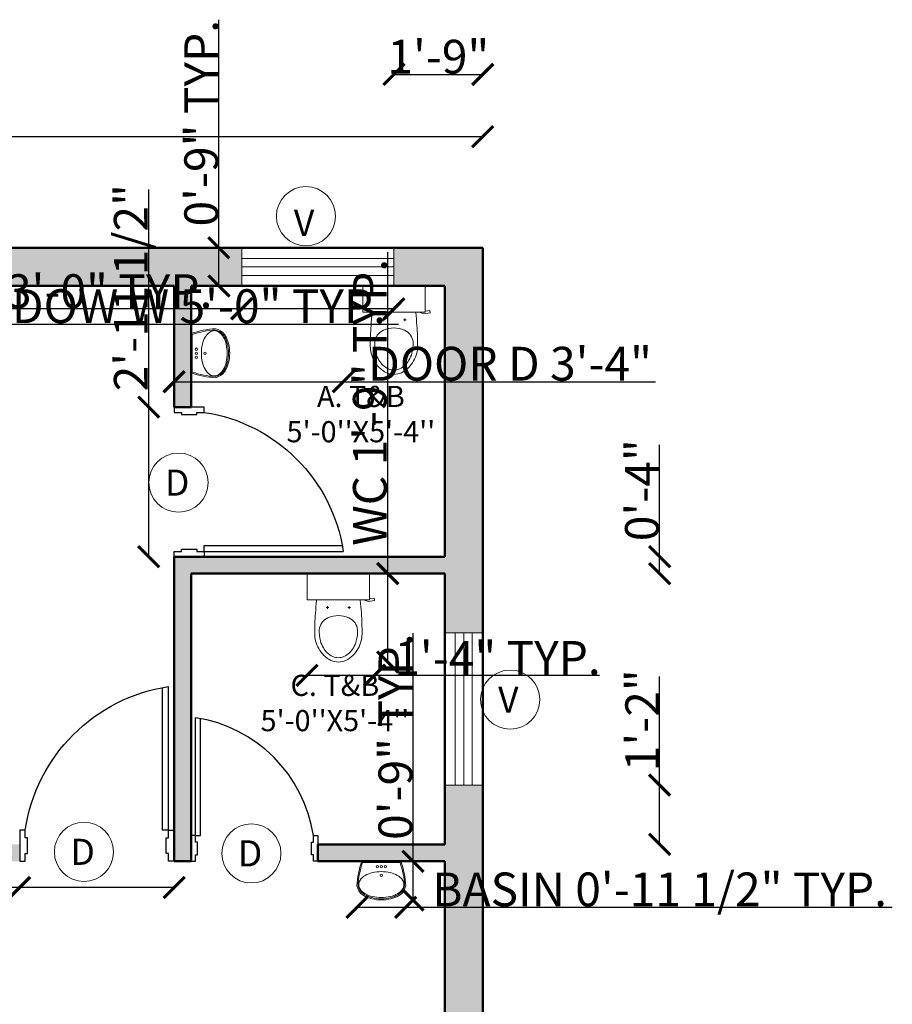
# Model space of a CAD drawing. Units: inches. Extents: x 1938 to 2373, y 1634 to 2225.
# Tile 5 of 5: x 2167 to 2373, y 1945 to 2178. Entities that reach past the tile are written whole.
import ezdxf

# ---------------------------------------------------------------- set-up
doc = ezdxf.new("R2010")
doc.units = ezdxf.units.IN
for name, color, linetype, lineweight in [('A-ANNO-DIMS', 2, 'Continuous', 18), ('A-ANNO-SYMB', 7, 'Continuous', 18), ('A-AREA-IDEN', 7, 'Continuous', 18), ('A-FLOR-FIXT', 9, 'Continuous', 18), ('A-WALL-PATT', 82, 'Continuous', 13), ('DOOR', 30, 'Continuous', 25), ('WALL', 7, 'Continuous', 50), ('WINDOW', 150, 'Continuous', 18)]:
    doc.layers.add(name, color=color, linetype=linetype, lineweight=lineweight)
doc.styles.get("Standard").update_dxf_attribs({"font": 'arial.ttf'})
doc.dimstyles.get("Standard").update_dxf_attribs({"dimtxt": 8, "dimasz": 5, "dimexe": 0.18, "dimexo": 0.0625, "dimgap": 0.09, "dimtad": 1, "dimdec": 1, "dimzin": 0, "dimdsep": 46, "dimlunit": 4, "dimtxsty": 'Standard', "dimblk": 'ARCHTICK', "dimcen": 0.09, "dimse1": 1, "dimse2": 1, "dimadec": 0, "dimazin": 0, "dimtfac": 1, "dimtdec": 1, "dimtofl": 0, "dimtmove": 0, "dimatfit": 3, "dimfxl": 1, "dimtolj": 1, "dimtzin": 0, "dimarcsym": 0})

# ---------------------------------------------------------------- blocks, each defined once
blk = doc.blocks.new('AP0B07')
for p, q in [((33.6, 96), (33.6, 978.8)), ((72, 96), (72, 972.3)), ((0, 96), (0, -96)), ((33.6, 96), (0, 96)), ((33.6, 48), (33.6, 96)), ((48, 48), (33.6, 48)), ((48, -48), (48, 48)), ((33.6, -96), (33.6, -48)), ((33.6, -48), (48, -48)), ((0, -96), (33.6, -96))]:
    blk.add_line(p, q)
blk.add_lwpolyline([(33.6, 96), (72, 96)])
blk.add_lwpolyline([(950, 96), (950, -96), (916.4, -96), (916.4, -48), (902, -48), (902, 48), (916.4, 48), (916.4, 96)], close=True)
blk.add_arc((-123.6, -61.2), 1051.8, 8.59637, 81.40363)
blk = doc.blocks.new('wash-3')
at = {"color": 0, "linetype": 'ByBlock'}
blk.add_line((0.23, -0.015), (-0.23, -0.015), dxfattribs=at)
for centre in [(-0.05, -0.066), (0, -0.066), (0.05, -0.066), (0, -0.172)]:
    blk.add_circle(centre, 0.0148, dxfattribs=at)
for centre, radius, start, end in [((0.69, -0.34), 0.991, 159.941, 177.839), ((0.69, -0.34), 0.976, 160.5399, 177.7326), ((-0.69, -0.34), 0.976, 2.2674, 19.4601), ((-0.69, -0.34), 0.991, 2.161, 20.059), ((-0.183, -0.286), 0.095, 144.1588, 180), ((-0.096, -0.349), 0.203, 119.8322, 144.1588), ((-0.038, -0.45), 0.319, 103.3619, 119.8322), ((0, -0.61), 0.483, 90, 103.3619), ((0, -0.61), 0.483, 76.6381, 90), ((0.038, -0.45), 0.319, 60.1678, 76.6381), ((0.096, -0.349), 0.203, 35.8412, 60.1678), ((0.183, -0.286), 0.095, 0, 35.8412), ((-0.12, -0.265), 0.184, 191.7424, 233.4191), ((-0.12, -0.265), 0.169, 192.3358, 233.361), ((-0.183, -0.286), 0.095, 180, 215.8412), ((-0.096, -0.223), 0.203, 215.8412, 240.1678), ((0.096, -0.223), 0.203, 299.8322, 324.1588), ((0.12, -0.265), 0.169, 306.639, 347.6642), ((0.12, -0.265), 0.184, 306.5809, 348.2576), ((0.183, -0.286), 0.095, 324.1588, 0), ((-0.096, -0.223), 0.232, 234.7719, 240.1678), ((-0.096, -0.223), 0.217, 234.8176, 240.1678), ((-0.038, -0.122), 0.348, 240.1678, 256.6381), ((-0.038, -0.122), 0.333, 240.1678, 256.6381), ((-0.038, -0.122), 0.319, 240.1678, 256.6381), ((0, 0.038), 0.513, 256.6381, 270), ((0, 0.038), 0.498, 256.6381, 270), ((0, 0.038), 0.483, 256.6381, 270), ((0, 0.038), 0.483, 270, 283.3619), ((0, 0.038), 0.498, 270, 283.3619), ((0, 0.038), 0.513, 270, 283.3619), ((0.038, -0.122), 0.319, 283.3619, 299.8322), ((0.038, -0.122), 0.333, 283.3619, 299.8322), ((0.038, -0.122), 0.348, 283.3619, 299.8322), ((0.096, -0.223), 0.217, 299.8322, 305.1824), ((0.096, -0.223), 0.232, 299.8322, 305.2281)]:
    blk.add_arc(centre, radius, start, end, dxfattribs=at)
blk = doc.blocks.new('toilet-1')
at = {"color": 0, "linetype": 'ByBlock'}
for p, q in [((-0.23, -0.02), (-0.23, -0.2116)), ((0.23, -0.02), (-0.23, -0.02)), ((0.23, -0.02), (0.23, -0.2116)), ((-0.23, -0.2116), (0.23, -0.2116)), ((0.1917, -0.2144), (0.2206, -0.225)), ((0.2633, -0.1997), (0.23, -0.2044)), ((0.266, -0.2187), (0.2633, -0.1997)), ((-0.0889, -0.2683), (-0.0697, -0.2683)), ((-0.0793, -0.2587), (-0.0793, -0.2778)), ((0.0889, -0.2683), (0.0698, -0.2683)), ((0.0794, -0.2587), (0.0794, -0.2778)), ((0.2206, -0.225), (0.266, -0.2187)), ((0, -0.6382), (0, -0.6382))]:
    blk.add_line(p, q, dxfattribs=at)
for centre, radius, start, end in [((3.5272, -0.6239), 3.7093, 173.69251, 175.15926), ((-3.527, -0.624), 3.7093, 4.84131, 6.31706), ((1.7368, -0.4519), 1.9109, 175.76982, 180.37578), ((-0.0312, -0.4465), 0.1114, 113.89968, 145.1485), ((0, -0.5169), 0.1884, 66.09393, 113.90607), ((0.0312, -0.4465), 0.1114, 34.8515, 66.10032), ((-1.7366, -0.4519), 1.9109, 359.62422, 4.23018), ((0.0981, -0.4497), 0.2389, 175.88621, 195.59308), ((-0.0408, -0.4398), 0.0996, 145.14967, 175.88096), ((0.0409, -0.4398), 0.0996, 4.11904, 34.85033), ((-0.098, -0.4497), 0.2389, 344.40692, 4.11379), ((0.0353, -0.463), 0.2093, 180.37466, 194.33753), ((-0.0351, -0.463), 0.2093, 345.6614, 359.62427), ((0.055, -0.458), 0.2297, 194.33532, 209.62204), ((0.0647, -0.4524), 0.2409, 209.62726, 224.54888), ((0.0961, -0.4503), 0.2369, 195.59686, 209.37705), ((0.0232, -0.4913), 0.1532, 209.38715, 226.54376), ((-0.0231, -0.4913), 0.1532, 313.45624, 330.61285), ((-0.0645, -0.4524), 0.2409, 315.45042, 330.37204), ((-0.096, -0.4503), 0.2369, 330.62295, 344.40314), ((-0.0548, -0.458), 0.2297, 330.37879, 345.66551), ((0.0178, -0.4986), 0.1751, 224.55199, 245.714), ((0.0152, -0.4997), 0.1416, 226.55015, 246.55272), ((0, -0.5347), 0.1034, 246.54933, 270.0042), ((0, -0.5347), 0.1034, 269.9958, 293.45067), ((-0.0151, -0.4997), 0.1416, 293.44728, 313.44985), ((-0.0176, -0.4986), 0.1751, 294.28649, 315.4485), ((0.0004, -0.538), 0.132, 245.58449, 269.87817), ((-0.0002, -0.538), 0.132, 270.12162, 294.4153)]:
    blk.add_arc(centre, radius, start, end, dxfattribs=at)
blk = doc.blocks.new('_ArchTick')
at = {"color": 0, "linetype": 'ByBlock', "const_width": 0.15}
blk.add_lwpolyline([(-0.5, -0.5), (0.5, 0.5)], dxfattribs=at)
blk = doc.blocks.new('*D12')
at = {"layer": 'A-ANNO-DIMS', "color": 0, "lineweight": -2, "transparency": 16777216}
blk.add_line((2000.23, 2149.88), (2276.23, 2149.88), dxfattribs=at)
at = {"layer": 'Defpoints', "color": 0, "transparency": 16777216}
for p in [(2276.23, 2149.88), (2000.23, 2123.59), (2276.23, 2123.59)]:
    blk.add_point(p, dxfattribs=at)
at = {"layer": 'A-ANNO-DIMS', "color": 0, "lineweight": -2, "transparency": 16777216, "xscale": 5, "yscale": 5, "zscale": 5, "rotation": 180}
blk.add_blockref('_ArchTick', (2000.23, 2149.88), dxfattribs=at)
at = {"layer": 'A-ANNO-DIMS', "color": 0, "lineweight": -2, "transparency": 16777216, "xscale": 5, "yscale": 5, "zscale": 5}
blk.add_blockref('_ArchTick', (2276.23, 2149.88), dxfattribs=at)
at = {"layer": 'A-ANNO-DIMS', "color": 0, "transparency": 16777216, "insert": (2138.23, 2154.06), "char_height": 8, "attachment_point": 5}
blk.add_mtext("\\A1;23'", dxfattribs=at)
blk = doc.blocks.new('VENT-36IN')
for p, q in [((2.5, 36), (2.5, 0)), ((4.5, 36), (4.5, 0)), ((6.5, 36), (6.5, 0))]:
    blk.add_line(p, q)
blk.add_lwpolyline([(9, 36), (0, 36), (0, 0), (9, 0)], close=True)
blk = doc.blocks.new('TAG-DOOR-D')
blk.add_circle((7, 7), 7)
blk.add_text('D', height=6.17).set_placement((3.79, 3.92))
blk = doc.blocks.new('*D21')
at = {"layer": 'A-ANNO-DIMS', "color": 0, "lineweight": -2, "transparency": 16777216}
for p, q in [((2160.51, 2019.91), (2160.51, 2112.41)), ((2160.51, 1978.59), (2160.51, 2019.91))]:
    blk.add_line(p, q, dxfattribs=at)
at = {"layer": 'Defpoints', "color": 0, "transparency": 16777216}
for p in [(2160.51, 2019.91), (2166.7, 2019.91), (2166.7, 1978.59)]:
    blk.add_point(p, dxfattribs=at)
at = {"layer": 'A-ANNO-DIMS', "color": 0, "lineweight": -2, "transparency": 16777216, "xscale": 5, "yscale": 5, "zscale": 5}
for p, rotation in [((2160.51, 2019.91), 90), ((2160.51, 1978.59), 270)]:
    blk.add_blockref('_ArchTick', p, dxfattribs=dict(at, rotation=rotation))
at = {"layer": 'A-ANNO-DIMS', "color": 0, "transparency": 16777216, "insert": (2156.27, 2068.66), "char_height": 8, "attachment_point": 5, "rotation": 90}
blk.add_mtext('\\A1;DOOR D 3\'-5 1/2"', dxfattribs=at)
blk = doc.blocks.new('*D22')
at = {"layer": 'A-ANNO-DIMS', "color": 0, "lineweight": -2, "transparency": 16777216}
for p, q in [((2166.7, 1972.39), (2121.62, 1972.39)), ((2203.23, 1972.39), (2166.7, 1972.39))]:
    blk.add_line(p, q, dxfattribs=at)
at = {"layer": 'Defpoints', "color": 0, "transparency": 16777216}
for p in [(2166.7, 1978.59), (2203.23, 1978.59), (2166.7, 1972.39)]:
    blk.add_point(p, dxfattribs=at)
at = {"layer": 'A-ANNO-DIMS', "color": 0, "lineweight": -2, "transparency": 16777216, "xscale": 5, "yscale": 5, "zscale": 5, "rotation": 180}
blk.add_blockref('_ArchTick', (2166.7, 1972.39), dxfattribs=at)
at = {"layer": 'A-ANNO-DIMS', "color": 0, "lineweight": -2, "transparency": 16777216, "xscale": 5, "yscale": 5, "zscale": 5}
blk.add_blockref('_ArchTick', (2203.23, 1972.39), dxfattribs=at)
at = {"layer": 'A-ANNO-DIMS', "color": 0, "transparency": 16777216, "insert": (2141.66, 1976.62), "char_height": 8, "attachment_point": 5}
blk.add_mtext('\\A1;3\'-0 1/2"', dxfattribs=at)
blk = doc.blocks.new('*D23')
at = {"layer": 'A-ANNO-DIMS', "color": 0, "lineweight": -2, "transparency": 16777216}
for p, q in [((2203.23, 2091.96), (2243.25, 2091.96)), ((2243.25, 2091.96), (2317.11, 2091.96))]:
    blk.add_line(p, q, dxfattribs=at)
at = {"layer": 'Defpoints', "color": 0, "transparency": 16777216}
for p in [(2243.25, 2091.96), (2203.23, 2085.96), (2243.25, 2085.96)]:
    blk.add_point(p, dxfattribs=at)
at = {"layer": 'A-ANNO-DIMS', "color": 0, "lineweight": -2, "transparency": 16777216, "xscale": 5, "yscale": 5, "zscale": 5, "rotation": 180}
blk.add_blockref('_ArchTick', (2203.23, 2091.96), dxfattribs=at)
at = {"layer": 'A-ANNO-DIMS', "color": 0, "lineweight": -2, "transparency": 16777216, "xscale": 5, "yscale": 5, "zscale": 5}
blk.add_blockref('_ArchTick', (2243.25, 2091.96), dxfattribs=at)
at = {"layer": 'A-ANNO-DIMS', "color": 0, "transparency": 16777216, "insert": (2282.68, 2096.2), "char_height": 8, "attachment_point": 5}
blk.add_mtext('\\A1;DOOR D 3\'-4"', dxfattribs=at)
blk = doc.blocks.new('*D24')
at = {"layer": 'A-ANNO-DIMS', "color": 0, "lineweight": -2, "transparency": 16777216}
for p, q in [((2197.23, 2085.96), (2197.23, 2137.4)), ((2197.23, 2050.59), (2197.23, 2085.96))]:
    blk.add_line(p, q, dxfattribs=at)
at = {"layer": 'Defpoints', "color": 0, "transparency": 16777216}
for p in [(2197.23, 2085.96), (2203.23, 2085.96), (2203.23, 2050.59)]:
    blk.add_point(p, dxfattribs=at)
at = {"layer": 'A-ANNO-DIMS', "color": 0, "lineweight": -2, "transparency": 16777216, "xscale": 5, "yscale": 5, "zscale": 5}
for p, rotation in [((2197.23, 2085.96), 90), ((2197.23, 2050.59), 270)]:
    blk.add_blockref('_ArchTick', p, dxfattribs=dict(at, rotation=rotation))
at = {"layer": 'A-ANNO-DIMS', "color": 0, "transparency": 16777216, "insert": (2193, 2114.18), "char_height": 8, "attachment_point": 5, "rotation": 90}
blk.add_mtext('\\A1;2\'-11 1/2"', dxfattribs=at)
blk = doc.blocks.new('*D29')
at = {"layer": 'A-ANNO-DIMS', "color": 0, "lineweight": -2, "transparency": 16777216}
for p, q in [((2076.23, 2105.59), (2136.23, 2105.59)), ((2136.23, 2105.59), (2256.3, 2105.59))]:
    blk.add_line(p, q, dxfattribs=at)
at = {"layer": 'Defpoints', "color": 0, "transparency": 16777216}
for p in [(2076.23, 2114.59), (2136.23, 2114.59), (2136.23, 2105.59)]:
    blk.add_point(p, dxfattribs=at)
at = {"layer": 'A-ANNO-DIMS', "color": 0, "lineweight": -2, "transparency": 16777216, "xscale": 5, "yscale": 5, "zscale": 5, "rotation": 180}
blk.add_blockref('_ArchTick', (2076.23, 2105.59), dxfattribs=at)
at = {"layer": 'A-ANNO-DIMS', "color": 0, "lineweight": -2, "transparency": 16777216, "xscale": 5, "yscale": 5, "zscale": 5}
blk.add_blockref('_ArchTick', (2136.23, 2105.59), dxfattribs=at)
at = {"layer": 'A-ANNO-DIMS', "color": 0, "transparency": 16777216, "insert": (2198.76, 2109.81), "char_height": 8, "attachment_point": 5}
blk.add_mtext('\\A1;WINDOW W 5\'-0" TYP.', dxfattribs=at)
blk = doc.blocks.new('*D33')
at = {"layer": 'A-ANNO-DIMS', "color": 0, "lineweight": -2, "transparency": 16777216}
for p, q in [((2246.47, 1967.71), (2258.01, 1967.71)), ((2258.01, 1967.71), (2373.1, 1967.71))]:
    blk.add_line(p, q, dxfattribs=at)
at = {"layer": 'Defpoints', "color": 0, "transparency": 16777216}
for p in [(2246.47, 1969.44), (2258.01, 1969.44), (2258.01, 1967.71)]:
    blk.add_point(p, dxfattribs=at)
at = {"layer": 'A-ANNO-DIMS', "color": 0, "lineweight": -2, "transparency": 16777216, "xscale": 5, "yscale": 5, "zscale": 5, "rotation": 180}
blk.add_blockref('_ArchTick', (2246.47, 1967.71), dxfattribs=at)
at = {"layer": 'A-ANNO-DIMS', "color": 0, "lineweight": -2, "transparency": 16777216, "xscale": 5, "yscale": 5, "zscale": 5}
blk.add_blockref('_ArchTick', (2258.01, 1967.71), dxfattribs=at)
at = {"layer": 'A-ANNO-DIMS', "color": 0, "transparency": 16777216, "insert": (2318.06, 1971.94), "char_height": 8, "attachment_point": 5}
blk.add_mtext('\\A1;BASIN 0\'-11 1/2" TYP.', dxfattribs=at)
blk = doc.blocks.new('*D34')
at = {"layer": 'A-ANNO-DIMS', "color": 0, "lineweight": -2, "transparency": 16777216}
for p, q in [((2259.74, 1978.59), (2259.74, 2032.53)), ((2259.74, 1969.44), (2259.74, 1978.59))]:
    blk.add_line(p, q, dxfattribs=at)
at = {"layer": 'Defpoints', "color": 0, "transparency": 16777216}
for p in [(2258.01, 1978.59), (2259.74, 1978.59), (2258.01, 1969.44)]:
    blk.add_point(p, dxfattribs=at)
at = {"layer": 'A-ANNO-DIMS', "color": 0, "lineweight": -2, "transparency": 16777216, "xscale": 5, "yscale": 5, "zscale": 5}
for p, rotation in [((2259.74, 1978.59), 90), ((2259.74, 1969.44), 270)]:
    blk.add_blockref('_ArchTick', p, dxfattribs=dict(at, rotation=rotation))
at = {"layer": 'A-ANNO-DIMS', "color": 0, "transparency": 16777216, "insert": (2255.57, 2008.06), "char_height": 8, "attachment_point": 5, "rotation": 90}
blk.add_mtext('\\A1;0\'-9" TYP.', dxfattribs=at)
blk = doc.blocks.new('*D37')
at = {"layer": 'A-ANNO-DIMS', "color": 0, "lineweight": -2, "transparency": 16777216}
for p, q in [((2253.76, 2046.59), (2253.76, 2122.58)), ((2253.76, 2025.69), (2253.76, 2046.59))]:
    blk.add_line(p, q, dxfattribs=at)
at = {"layer": 'Defpoints', "color": 0, "transparency": 16777216}
for p in [(2250.63, 2046.59), (2253.76, 2046.59), (2250.63, 2025.69)]:
    blk.add_point(p, dxfattribs=at)
at = {"layer": 'A-ANNO-DIMS', "color": 0, "lineweight": -2, "transparency": 16777216, "xscale": 5, "yscale": 5, "zscale": 5}
for p, rotation in [((2253.76, 2046.59), 90), ((2253.76, 2025.69), 270)]:
    blk.add_blockref('_ArchTick', p, dxfattribs=dict(at, rotation=rotation))
at = {"layer": 'A-ANNO-DIMS', "color": 0, "transparency": 16777216, "insert": (2249.54, 2087.08), "char_height": 8, "attachment_point": 5, "rotation": 90}
blk.add_mtext('\\A1;WC 1\'-9" TYP.', dxfattribs=at)
blk = doc.blocks.new('*D38')
at = {"layer": 'A-ANNO-DIMS', "color": 0, "lineweight": -2, "transparency": 16777216}
for p, q in [((2234.68, 2022.55), (2250.63, 2022.55)), ((2250.63, 2022.55), (2303.82, 2022.55))]:
    blk.add_line(p, q, dxfattribs=at)
at = {"layer": 'Defpoints', "color": 0, "transparency": 16777216}
for p in [(2234.68, 2025.69), (2250.63, 2025.69), (2250.63, 2022.55)]:
    blk.add_point(p, dxfattribs=at)
at = {"layer": 'A-ANNO-DIMS', "color": 0, "lineweight": -2, "transparency": 16777216, "xscale": 5, "yscale": 5, "zscale": 5, "rotation": 180}
blk.add_blockref('_ArchTick', (2234.68, 2022.55), dxfattribs=at)
at = {"layer": 'A-ANNO-DIMS', "color": 0, "lineweight": -2, "transparency": 16777216, "xscale": 5, "yscale": 5, "zscale": 5}
blk.add_blockref('_ArchTick', (2250.63, 2022.55), dxfattribs=at)
at = {"layer": 'A-ANNO-DIMS', "color": 0, "transparency": 16777216, "insert": (2279.72, 2026.66), "char_height": 8, "attachment_point": 5}
blk.add_mtext('\\A1;1\'-4" TYP.', dxfattribs=at)
blk = doc.blocks.new('*D41')
at = {"layer": 'A-ANNO-DIMS', "color": 0, "lineweight": -2, "transparency": 16777216}
for p, q in [((2219.23, 2109.19), (2131.96, 2109.19)), ((2255.23, 2109.19), (2219.23, 2109.19))]:
    blk.add_line(p, q, dxfattribs=at)
at = {"layer": 'Defpoints', "color": 0, "transparency": 16777216}
for p in [(2219.23, 2114.59), (2255.23, 2114.59), (2219.23, 2109.19)]:
    blk.add_point(p, dxfattribs=at)
at = {"layer": 'A-ANNO-DIMS', "color": 0, "lineweight": -2, "transparency": 16777216, "xscale": 5, "yscale": 5, "zscale": 5}
for p, rotation in [((2219.23, 2109.19), 179.9999999999986), ((2255.23, 2109.19), 359.9999999999986)]:
    blk.add_blockref('_ArchTick', p, dxfattribs=dict(at, rotation=rotation))
at = {"layer": 'A-ANNO-DIMS', "color": 0, "transparency": 16777216, "insert": (2173.09, 2113.36), "char_height": 8, "attachment_point": 5}
blk.add_mtext('\\A1;VENT 3\'-0" TYP.', dxfattribs=at)
blk = doc.blocks.new('*D42')
at = {"layer": 'A-ANNO-DIMS', "color": 0, "lineweight": -2, "transparency": 16777216}
for p, q in [((2213.83, 2123.59), (2213.83, 2177.53)), ((2213.83, 2114.59), (2213.83, 2123.59))]:
    blk.add_line(p, q, dxfattribs=at)
at = {"layer": 'Defpoints', "color": 0, "transparency": 16777216}
for p in [(2213.83, 2123.59), (2219.23, 2123.59), (2219.23, 2114.59)]:
    blk.add_point(p, dxfattribs=at)
at = {"layer": 'A-ANNO-DIMS', "color": 0, "lineweight": -2, "transparency": 16777216, "xscale": 5, "yscale": 5, "zscale": 5}
for p, rotation in [((2213.83, 2123.59), 90), ((2213.83, 2114.59), 270)]:
    blk.add_blockref('_ArchTick', p, dxfattribs=dict(at, rotation=rotation))
at = {"layer": 'A-ANNO-DIMS', "color": 0, "transparency": 16777216, "insert": (2209.65, 2153.06), "char_height": 8, "attachment_point": 5, "rotation": 90}
blk.add_mtext('\\A1;0\'-9" TYP.', dxfattribs=at)
blk = doc.blocks.new('*D59')
at = {"layer": 'A-ANNO-DIMS', "color": 0, "lineweight": -2, "transparency": 16777216}
blk.add_line((2255.23, 2164.6), (2276.23, 2164.6), dxfattribs=at)
at = {"layer": 'Defpoints', "color": 0, "transparency": 16777216}
for p in [(2276.23, 2164.6), (2255.23, 2123.59), (2276.23, 2123.59)]:
    blk.add_point(p, dxfattribs=at)
at = {"layer": 'A-ANNO-DIMS', "color": 0, "lineweight": -2, "transparency": 16777216, "xscale": 5, "yscale": 5, "zscale": 5, "rotation": 180}
blk.add_blockref('_ArchTick', (2255.23, 2164.6), dxfattribs=at)
at = {"layer": 'A-ANNO-DIMS', "color": 0, "lineweight": -2, "transparency": 16777216, "xscale": 5, "yscale": 5, "zscale": 5}
blk.add_blockref('_ArchTick', (2276.23, 2164.6), dxfattribs=at)
at = {"layer": 'A-ANNO-DIMS', "color": 0, "transparency": 16777216, "insert": (2265.73, 2168.77), "char_height": 8, "attachment_point": 5}
blk.add_mtext('\\A1;1\'-9"', dxfattribs=at)
blk = doc.blocks.new('*D64')
at = {"layer": 'A-ANNO-DIMS', "color": 0, "lineweight": -2, "transparency": 16777216}
for p, q in [((2318.07, 1996.59), (2318.07, 2022.28)), ((2318.07, 1982.59), (2318.07, 1996.59))]:
    blk.add_line(p, q, dxfattribs=at)
at = {"layer": 'Defpoints', "color": 0, "transparency": 16777216}
for p in [(2267.23, 1996.59), (2318.07, 1996.59), (2267.23, 1982.59)]:
    blk.add_point(p, dxfattribs=at)
at = {"layer": 'A-ANNO-DIMS', "color": 0, "lineweight": -2, "transparency": 16777216, "xscale": 5, "yscale": 5, "zscale": 5}
for p, rotation in [((2318.07, 1996.59), 90), ((2318.07, 1982.59), 270)]:
    blk.add_blockref('_ArchTick', p, dxfattribs=dict(at, rotation=rotation))
at = {"layer": 'A-ANNO-DIMS', "color": 0, "transparency": 16777216, "insert": (2313.96, 2011.93), "char_height": 8, "attachment_point": 5, "rotation": 90}
blk.add_mtext('\\A1;1\'-2"', dxfattribs=at)
blk = doc.blocks.new('*D66')
at = {"layer": 'A-ANNO-DIMS', "color": 0, "lineweight": -2, "transparency": 16777216}
for p, q in [((2318.07, 2050.59), (2318.07, 2077.03)), ((2318.07, 2046.59), (2318.07, 2050.59))]:
    blk.add_line(p, q, dxfattribs=at)
at = {"layer": 'Defpoints', "color": 0, "transparency": 16777216}
for p in [(2267.23, 2050.59), (2318.07, 2050.59), (2267.23, 2046.59)]:
    blk.add_point(p, dxfattribs=at)
at = {"layer": 'A-ANNO-DIMS', "color": 0, "lineweight": -2, "transparency": 16777216, "xscale": 5, "yscale": 5, "zscale": 5}
for p, rotation in [((2318.07, 2050.59), 90), ((2318.07, 2046.59), 270)]:
    blk.add_blockref('_ArchTick', p, dxfattribs=dict(at, rotation=rotation))
at = {"layer": 'A-ANNO-DIMS', "color": 0, "transparency": 16777216, "insert": (2313.89, 2066.31), "char_height": 8, "attachment_point": 5, "rotation": 90}
blk.add_mtext('\\A1;0\'-4"', dxfattribs=at)

msp = doc.modelspace()

# ---------------------------------------------------------------- hatches: boundary and pattern name
at = {"layer": 'A-WALL-PATT', "transparency": 33554585}
h = msp.add_hatch(color=256, dxfattribs=at)
h.dxf.hatch_style = 1
h.paths.add_polyline_path([(2076.23, 2123.59), (2000.23, 2123.59), (2000.23, 2078.59), (2009.23, 2078.59), (2009.23, 2078.85), (2009.23, 2114.59), (2076.23, 2114.59)])
h.paths.add_polyline_path([(2219.23, 2123.59), (2136.23, 2123.59), (2136.23, 2114.59), (2203.23, 2114.59), (2203.23, 2085.96), (2207.23, 2085.96), (2207.23, 2114.59), (2219.23, 2114.59)])
h.paths.add_polyline_path([(2276.23, 2123.59), (2255.23, 2123.59), (2255.23, 2114.59), (2262.62, 2114.59), (2267.23, 2114.59), (2267.23, 2050.59), (2203.23, 2050.59), (2203.23, 1978.59), (2207.23, 1978.59), (2207.23, 1984.65), (2207.23, 2046.59), (2267.23, 2046.59), (2267.23, 2032.59), (2276.23, 2032.59)])
h.paths.add_polyline_path([(2009.23, 2018.59), (2000.23, 2018.59), (2000.23, 1948.59), (2009.23, 1948.59), (2009.23, 1948.85), (2009.23, 1978.59), (2126.4, 1978.59), (2126.4, 1978.59), (2133.23, 1978.59), (2166.7, 1978.59), (2166.7, 1982.59), (2009.23, 1982.59)])
h.paths.add_polyline_path([(2276.23, 1996.59), (2267.23, 1996.59), (2267.23, 1982.59), (2237.23, 1982.59), (2237.23, 1978.59), (2267.23, 1978.59), (2267.23, 1901.32), (2276.23, 1901.32)])
h.paths.add_polyline_path([(2133.23, 1944.79), (2129.23, 1944.79), (2129.23, 1858.59), (2009.23, 1858.59), (2009.23, 1888.59), (2000.23, 1888.59), (2000.23, 1839.09), (2009.23, 1839.09), (2009.23, 1854.59), (2091.31, 1854.59), (2091.31, 1854.61), (2097.36, 1854.59), (2133.23, 1854.59)])
h.paths.add_polyline_path([(2121.02, 1763.59), (2097.23, 1763.59), (2097.23, 1824.61), (2093.23, 1824.61), (2093.23, 1763.59), (2009.23, 1763.59), (2009.23, 1779.09), (2000.23, 1779.09), (2000.23, 1739.59), (2009.23, 1739.59), (2009.23, 1754.59), (2121.02, 1754.59)])
h.paths.add_polyline_path([(2108.23, 1676.59), (2009.23, 1676.59), (2009.23, 1691.59), (2000.23, 1691.59), (2000.23, 1667.59), (2108.23, 1667.59)])
h.paths.add_polyline_path([(2276.23, 1841.32), (2267.23, 1841.32), (2267.23, 1763.59), (2246.64, 1763.59), (2246.64, 1754.59), (2276.23, 1754.59)])

# ---------------------------------------------------------------- linework, layer by layer
at = {"layer": 'A-ANNO-SYMB'}
for centre in [(2234.41, 2131.07), (2282.72, 2016.8)]:
    msp.add_circle(centre, 7, dxfattribs=at)
at = {"layer": 'WALL'}
for p, q in [((2000.23, 2123.59), (2276.23, 2123.59)), ((2276.23, 2123.59), (2276.23, 1667.59)), ((2009.23, 2114.59), (2203.23, 2114.59)), ((2203.23, 2114.59), (2203.23, 2085.96)), ((2207.23, 2114.59), (2207.23, 2085.96)), ((2207.23, 2114.59), (2267.23, 2114.59)), ((2267.23, 2114.59), (2267.23, 2050.59)), ((2203.23, 2085.96), (2207.23, 2085.96)), ((2203.23, 2050.59), (2267.23, 2050.59)), ((2203.23, 2050.59), (2203.23, 1978.59)), ((2207.23, 2046.59), (2267.23, 2046.59)), ((2207.23, 2046.59), (2207.23, 1978.59)), ((2267.23, 2046.59), (2267.23, 1982.59)), ((2237.23, 1982.59), (2267.23, 1982.59)), ((2237.23, 1982.59), (2237.23, 1978.59)), ((2203.23, 1978.59), (2207.23, 1978.59)), ((2237.23, 1978.59), (2267.23, 1978.59)), ((2267.23, 1763.59), (2267.23, 1978.59))]:
    msp.add_line(p, q, dxfattribs=at)

# ---------------------------------------------------------------- block references
at = {"layer": 'A-ANNO-SYMB'}
for p in [(2197.27, 2061.1), (2174.91, 1973.82), (2214.5, 1973.46)]:
    msp.add_blockref('TAG-DOOR-D', p, dxfattribs=at)
at = {"layer": 'A-FLOR-FIXT'}
for name, p, xscale, yscale, zscale in [('toilet-1', (2255.23, 2115.23), 32.14984283332795, 32.14984283332795, 32.14984283332795), ('toilet-1', (2242.08, 2047.23), 32.14984283332795, 32.14984283332795, 32.14984283332795), ('wash-3', (2252.24, 1978.59), 19.24466160509284, 19.24466160509284, 19.24466160509284)]:
    msp.add_blockref(name, p, dxfattribs=dict(at, xscale=xscale, yscale=yscale, zscale=zscale))
at = {"layer": 'A-FLOR-FIXT', "xscale": 19.24466160509284, "yscale": 19.24466160509284, "zscale": 19.24466160509284, "rotation": 90}
msp.add_blockref('wash-3', (2207.23, 2098.68), dxfattribs=at)
at = {"layer": 'DOOR', "xscale": -0.0372377324197297, "yscale": 0.0372377324197297, "zscale": 0.0372377324197297, "rotation": 270}
msp.add_blockref('AP0B07', (2206.8, 2050.59), dxfattribs=at)
at = {"layer": 'DOOR'}
for p, xscale, yscale, zscale in [((2203.23, 1982.28), -0.0384472811899697, 0.0384472811899697, 0.0384472811899697), ((2207.23, 1981.62), 0.031578947368421, 0.031578947368421, 0.031578947368421)]:
    msp.add_blockref('AP0B07', p, dxfattribs=dict(at, xscale=xscale, yscale=yscale, zscale=zscale))
at = {"layer": 'WINDOW', "rotation": 89.99999999999844}
msp.add_blockref('VENT-36IN', (2255.23, 2114.59), dxfattribs=at)
at = {"layer": 'WINDOW'}
msp.add_blockref('VENT-36IN', (2267.23, 1996.59), dxfattribs=at)

# ---------------------------------------------------------------- texts
at = {"layer": 'A-ANNO-SYMB'}
for p in [(2231.55, 2126.42), (2279.86, 2013.72)]:
    msp.add_text('V', height=6.17, dxfattribs=at).set_placement(p)
at = {"layer": 'A-AREA-IDEN', "char_height": 5, "attachment_point": 1}
for s, insert in [("\\pxi-3,l4,qc,t4;A. T&B\\P5'-0''X5'-4''", (2213.15, 2090.97)), ("\\pxqc;C. T&B\\P5'-0''X5'-4''", (2209.5, 2022.68))]:
    msp.add_mtext_dynamic_manual_height_columns(s, width=63.5129, gutter_width=30.83, heights=[0], dxfattribs=dict(at, insert=insert))

# ---------------------------------------------------------------- dimensions: what is measured, and where the dimension line sits
at = {"layer": 'A-ANNO-DIMS'}
for base, p1, p2, angle, text, picture, middle in [((2213.83, 2123.59), (2219.23, 2114.59), (2219.23, 2123.59), 90, '<> TYP.', '*D42', (2209.65, 2153.06)), ((2136.23, 2105.59), (2076.23, 2114.59), (2136.23, 2114.59), 0, 'WINDOW W <> TYP.', '*D29', (2198.76, 2109.81)), ((2219.23, 2109.19), (2255.23, 2114.59), (2219.23, 2114.59), 180, 'VENT <> TYP.', '*D41', (2173.09, 2113.36)), ((2253.76, 2046.59), (2250.63, 2025.69), (2250.63, 2046.59), 90, 'WC <> TYP.', '*D37', (2249.54, 2087.08)), ((2160.51, 2019.91), (2166.7, 1978.59), (2166.7, 2019.91), 90, 'DOOR D <>', '*D21', (2156.27, 2068.66)), ((2259.7448, 1978.5853), (2258.0127, 1969.444), (2258.0127, 1978.5853), 90, '<> TYP.', '*D34', (2255.5702, 2008.0573))]:
    dim = msp.add_linear_dim(base=base, p1=p1, p2=p2, angle=angle, text=text, dimstyle='Standard', override={"dimdec": 1, "dimlfac": 1, "dimrnd": 0, "dimzin": 1, "dimdsep": 46, "dimlunit": 4, "dimfrac": 2}, dxfattribs=at)
    dim.commit()
    dim.dimension.update_dxf_attribs({"geometry": picture, "text_midpoint": middle})
for base, p1, override, picture, middle in [((2276.23, 2164.6), (2255.23, 2123.59), {"dimdec": 1, "dimlfac": 1, "dimrnd": 0, "dimzin": 1, "dimdsep": 46, "dimlunit": 4, "dimfrac": 2}, '*D59', (2265.73, 2168.77)), ((2276.23, 2149.88), (2000.23, 2123.59), {"dimclrd": 0, "dimclre": 0, "dimclrt": 0}, '*D12', (2138.23, 2154.06))]:
    dim = msp.add_linear_dim(base=base, p1=p1, p2=(2276.23, 2123.59), dimstyle='Standard', override=override, dxfattribs=at)
    dim.commit()
    dim.dimension.update_dxf_attribs({"geometry": picture, "text_midpoint": middle})
for base, p1, p2, angle, picture, middle in [((2197.23, 2085.96), (2203.23, 2050.59), (2203.23, 2085.96), 90, '*D24', (2193, 2114.18)), ((2318.07, 2050.59), (2267.23, 2046.59), (2267.23, 2050.59), 90, '*D66', (2313.89, 2066.31)), ((2318.07, 1996.59), (2267.23, 1982.59), (2267.23, 1996.59), 90, '*D64', (2313.96, 2011.93)), ((2166.7, 1972.39), (2203.23, 1978.59), (2166.7, 1978.59), 180, '*D22', (2141.66, 1976.62))]:
    dim = msp.add_linear_dim(base=base, p1=p1, p2=p2, angle=angle, dimstyle='Standard', override={"dimdec": 1, "dimlfac": 1, "dimrnd": 0, "dimzin": 1, "dimdsep": 46, "dimlunit": 4, "dimfrac": 2}, dxfattribs=at)
    dim.commit()
    dim.dimension.update_dxf_attribs({"geometry": picture, "text_midpoint": middle})
for base, p1, p2, text, picture, middle in [((2243.25, 2091.96), (2203.23, 2085.96), (2243.25, 2085.96), 'DOOR D <>', '*D23', (2282.68, 2096.2)), ((2250.6278, 2022.5533), (2234.6814, 2025.6879), (2250.6278, 2025.6879), '<> TYP.', '*D38', (2279.7232, 2026.6624)), ((2258.01, 1967.71), (2246.47, 1969.44), (2258.01, 1969.44), 'BASIN <> TYP.', '*D33', (2318.06, 1971.94))]:
    dim = msp.add_linear_dim(base=base, p1=p1, p2=p2, text=text, dimstyle='Standard', override={"dimdec": 1, "dimlfac": 1, "dimrnd": 0, "dimzin": 1, "dimdsep": 46, "dimlunit": 4, "dimfrac": 2}, dxfattribs=at)
    dim.commit()
    dim.dimension.update_dxf_attribs({"geometry": picture, "text_midpoint": middle})

doc.saveas('drawing.dxf')
